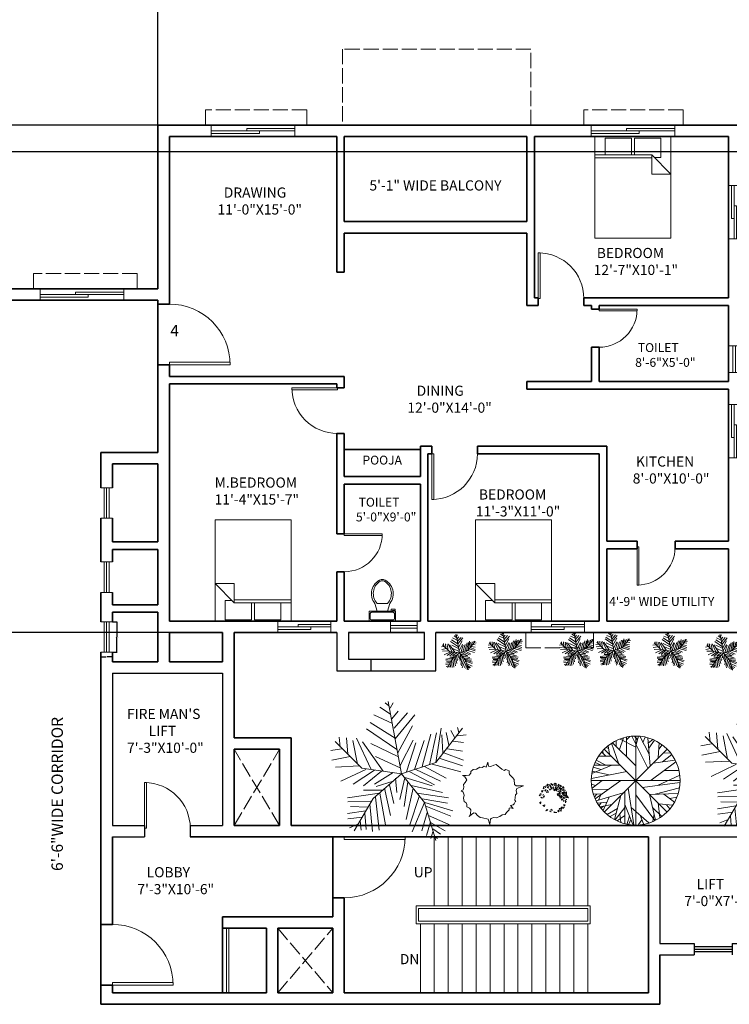
# Model space of a CAD drawing. Units: inches. Extents: x -69 to 2453, y 4803 to 7122.
# Tile 3 of 9: x 643 to 1203, y 5467 to 6243. Entities that reach past the tile are written whole.
import ezdxf

# ---------------------------------------------------------------- set-up
doc = ezdxf.new("R2010")
doc.units = ezdxf.units.IN
doc.linetypes.add('ACAD_ISO02W100', pattern=[15, 12, -3])
for name, color, linetype, lineweight in [('A-ANNO-DIMS', 2, 'Continuous', 18), ('A-ANNO-IDEN', 2, 'Continuous', 18), ('A-ANNO-TEXT', 7, 'Continuous', 18), ('A-AREA-IDEN', 7, 'Continuous', 18), ('A-DOOR', 3, 'Continuous', 18), ('A-FLOR-EVTR', 4, 'Continuous', 25), ('A-FLOR-FIXT', 9, 'Continuous', 18), ('A-FLOR-OPEN', 8, 'ACAD_ISO02W100', 13), ('A-FLOR-OVHD', 8, 'ACAD_ISO02W100', 13), ('A-FLOR-STRS', 4, 'Continuous', 18), ('A-FURN', 8, 'Continuous', 18), ('A-GLAZ', 244, 'Continuous', 18), ('A-WALL', 7, 'Continuous', 35), ('A-WALL-SRVC', 7, 'Continuous', 30), ('L-PLNT', 94, 'Continuous', 13)]:
    doc.layers.add(name, color=color, linetype=linetype, lineweight=lineweight)
doc.styles.get("Standard").update_dxf_attribs({"font": 'arial.ttf'})
doc.dimstyles.get("Standard").update_dxf_attribs({"dimtxt": 0.18, "dimasz": 0.18, "dimexe": 0.18, "dimexo": 0.0625, "dimgap": 0.09, "dimtad": 0, "dimtih": 1, "dimtoh": 1, "dimdec": 4, "dimzin": 0, "dimdsep": 46, "dimtxsty": 'Standard', "dimcen": 0.09, "dimadec": 0, "dimazin": 0, "dimtfac": 1, "dimtdec": 4, "dimtofl": 0, "dimtmove": 0, "dimatfit": 3, "dimfxl": 1, "dimtolj": 1, "dimtzin": 0, "dimarcsym": 0})

# ---------------------------------------------------------------- blocks, each defined once
blk = doc.blocks.new('*U7')
for p, q in [((0, 0), (0, -6)), ((-40, 0), (-40, -6))]:
    blk.add_line(p, q)
blk.add_lwpolyline([(0, 0), (0, 40), (-1.75, 40), (-1.75, 0)], close=True)
blk.add_arc((0, 0), 40, 90, 180)
blk = doc.blocks.new('*U5')
for p, q in [((0, 0), (0, -6)), ((40, 0), (40, -6))]:
    blk.add_line(p, q)
blk.add_lwpolyline([(0, 0), (0, 40), (1.75, 40), (1.75, 0)], close=True)
blk.add_arc((0, 0), 40, 0, 90)
blk = doc.blocks.new('*U4')
for p, q in [((0, 0), (0, -6)), ((-40, 0), (-40, -6))]:
    blk.add_line(p, q)
blk.add_lwpolyline([(0, 0), (0, 40), (-1.75, 40), (-1.75, 0)], close=True)
blk.add_arc((0, 0), 40, 90, 180)
blk = doc.blocks.new('*U3')
for p, q in [((0, 0), (0, 6)), ((40, 0), (40, 6))]:
    blk.add_line(p, q)
blk.add_lwpolyline([(0, 0), (0, -40), (1.75, -40), (1.75, 0)], close=True)
blk.add_arc((0, 0), 40, 270, 360)
blk = doc.blocks.new('*U8')
for p, q in [((0, 0), (0, 6)), ((40, 0), (40, 6))]:
    blk.add_line(p, q)
blk.add_lwpolyline([(0, 0), (0, -40), (1.75, -40), (1.75, 0)], close=True)
blk.add_arc((0, 0), 40, 270, 0)
blk = doc.blocks.new('*U21')
for p, q in [((-40, 0), (-40, -6)), ((0, 0), (0, -6))]:
    blk.add_line(p, q)
blk.add_lwpolyline([(0, 0), (0, 40), (-1.75, 40), (-1.75, 0)], close=True)
blk.add_arc((0, 0), 40, 90, 180)
blk = doc.blocks.new('*U23')
for p, q in [((0, 0), (0, -6)), ((40, 0), (40, -6))]:
    blk.add_line(p, q)
blk.add_lwpolyline([(0, 0), (0, 40), (1.75, 40), (1.75, 0)], close=True)
blk.add_arc((0, 0), 40, 0, 90)
blk = doc.blocks.new('*U27')
for points in [[(-5.78, 9.75), (-7.54, 9.23), (-8.01, 7.5), (-6.26, 8.45)], [(-4.43, 11.05), (-5.18, 10.36), (-3.96, 9.49), (-2.07, 10.36)], [(-4.84, 8.63), (-3.83, 7.85), (-4.03, 8.97)], [(-1.94, 9.49), (-2.48, 8.97), (-2.27, 8.54), (-1.8, 9.06)], [(-2, 11.66), (-1.6, 10.62), (-0.52, 10.1), (-0.18, 10.62), (-0.79, 10.96)], [(0.02, 9.06), (-1.33, 8.54), (-1.73, 7.16), (0.29, 7.76)], [(1.24, 12), (0.56, 11.31), (0.76, 10.01), (2.52, 11.05)], [(1.37, 8.54), (3.13, 8.8), (3.8, 7.85), (1.91, 7.76)], [(2.59, 9.93), (1.84, 9.75), (1.64, 9.23), (2.32, 9.41)], [(4.14, 11.14), (3.6, 10.01), (4, 9.23), (5.22, 8.71), (6.3, 9.41), (5.08, 10.19), (4.61, 10.01)], [(4.61, 8.28), (4.54, 7.76), (4.95, 7.59), (4.95, 8.28)], [(6.43, 7.94), (5.49, 7.68), (5.56, 6.21), (6.5, 6.64)], [(7.45, 9.32), (7.11, 7.94), (8.52, 7.94)], [(-11.32, 1.79), (-9.83, 2.31), (-9.63, 3.44), (-10.44, 3.52)], [(-8.21, 0.41), (-9.43, 0.32), (-9.83, 0.84)], [(-8.14, 6.03), (-9.36, 5.95), (-9.02, 4.73)], [(-8.21, 3.09), (-8.48, 2.31), (-7.87, 2.57)], [(-7, 1.79), (-7.94, 1.53), (-7.47, 0.49)], [(-5.78, 6.81), (-6.66, 6.21), (-6.52, 5.69)], [(-4.57, 6.38), (-5.45, 4.47), (-3.89, 4.82)], [(-2.88, 7.5), (-3.15, 6.64), (-2.27, 6.72)], [(0.76, 7.16), (0.09, 6.46), (1.1, 5.95)], [(1.71, 6.29), (1.71, 7.07), (2.65, 7.5), (2.11, 6.9)], [(2.52, 6.81), (2.52, 5.86), (4.41, 5.17), (4.61, 6.72)], [(3.53, 1.88), (2.86, 3.52), (3.8, 3.52)], [(4.41, 4.56), (4.27, 3.7), (5.49, 3.26)], [(4.27, 2.74), (5.29, 2.66), (4.41, 1.27)], [(5.83, 1.53), (5.02, 0.41), (5.49, -0.02), (6.5, 0.41)], [(5.49, 5.51), (5.42, 4.82), (6.16, 5.08)], [(7.51, 1.71), (6.91, 1.27), (6.23, 2.14)], [(8.12, 4.99), (7.11, 4.65), (6.5, 4.13), (7.38, 3.09), (8.12, 3.52), (7.65, 3.87)], [(7.85, 6.81), (7.18, 6.21), (9, 5.51), (9.33, 6.38)], [(8.12, 0.75), (7.51, 0.15), (8.93, -0.28), (9.13, 0.49)], [(8.19, 2.57), (7.92, 2.05), (8.66, 1.53)], [(8.73, 4.73), (8.19, 4.56), (8.39, 3.87), (8.59, 4.04)], [(10.28, 5.17), (9.2, 4.04), (9, 2.31), (10.48, 0.49), (11.76, 0.41), (10.35, 2.48), (9.33, 2.4), (10.28, 2.83)], [(-10.03, -2.71), (-10.64, -3.31), (-10.44, -4.44), (-9.9, -3.49)], [(-8.28, -5.73), (-6.79, -5.3), (-7, -6.51)], [(6.1, -8.94), (6.16, -7.21), (6.91, -6.69), (7.24, -7.38)], [(7.78, -0.8), (6.43, -1.5), (6.43, -0.72)], [(8.32, -1.75), (7.98, -2.53), (7.58, -2.1)], [(8.05, -8.07), (8.59, -7.12), (7.92, -7.55)], [(9.33, -5.13), (8.46, -6.25), (7.98, -5.22)], [(9.33, -1.75), (9.54, -3.74), (10.14, -2.53)], [(10.08, -0.63), (9.74, -1.32), (10.48, -0.89)], [(-4.84, -8.85), (-4.43, -9.45), (-5.99, -9.8)], [(-2.54, -10.06), (-3.02, -10.23), (-1.8, -10.67)], [(-2.34, -9.2), (-1.26, -8.5), (-0.99, -9.54)], [(0.22, -10.58), (0.83, -11.27), (2.59, -11.36)], [(4.07, -9.45), (3.53, -9.97), (4.07, -10.58), (4.61, -9.89)], [(5.29, -7.98), (4.61, -8.16), (5.02, -8.94)], [(6.03, -9.45), (5.42, -9.97), (6.16, -10.15)]]:
    blk.add_lwpolyline(points, close=True)
blk = doc.blocks.new('*U25')
for p, q in [((-10.186, 53.64), (-13.084, 55.962)), ((0, 0), (-10.5, 57)), ((-9.099, 51.782), (-6.563, 55.962)), ((-7.288, 39.707), (-21.778, 46.673)), ((-8.737, 47.138), (-17.069, 52.711)), ((-7.65, 43.423), (-2.578, 49.46)), ((-5.839, 35.992), (4.667, 48.067)), ((-5.114, 27.632), (10.463, 46.673)), ((-5.114, 28.097), (-24.676, 40.636)), ((-3.665, 19.273), (-27.574, 35.527)), ((-2.941, 16.486), (8.652, 37.85)), ((16.259, 5.805), (23.142, 31.348)), ((22.055, 7.198), (27.489, 32.277)), ((27, 9), (48, 36)), ((27.127, 9.056), (31.112, 35.992)), ((35.096, 32.741), (37.27, 22.524)), ((38.719, 34.134), (41.979, 28.561)), ((44.153, 36.456), (45.239, 32.741)), ((-31.5, 4.5), (-52.5, 25.5)), ((-48.585, 21.131), (-49.309, 29.026)), ((-43.513, 28.561), (-42.427, 15.558)), ((-38.442, 26.239), (-34.819, 7.663)), ((-35.544, 28.097), (-24.314, 3.947)), ((-14.533, 2.09), (-30.834, 25.31)), ((-24.314, 23.917), (-2.941, 13.7)), ((-1.129, 6.734), (9.014, 26.704)), ((3.942, 1.625), (11.187, 24.381)), ((10.101, 3.483), (17.708, 26.239)), ((31.836, 30.883), (32.561, 16.486)), ((40.53, 25.775), (48.862, 24.846)), ((43.791, 29.954), (51.036, 30.883)), ((-47.498, 19.737), (-55.83, 18.344)), ((33.285, 16.486), (48.862, 10.913)), ((36.183, 19.737), (48.137, 17.88)), ((-40.615, 13.7), (-55.105, 10.913)), ((-20.691, 13.7), (-1.129, 4.876)), ((0, 0), (27, 9)), ((29.662, 12.307), (48.137, 6.269)), ((-33.37, 6.269), (-52.207, 5.34)), ((-28.299, 3.483), (-47.86, -5.805)), ((-21.416, 3.018), (-38.079, -8.128)), ((0, 0), (-31.5, 4.5)), ((-15.982, 2.09), (-30.11, -9.521)), ((0, 0), (-22.5, -19.5)), ((-6.563, 1.161), (-21.416, -8.128)), ((0, 0), (18, -22.5)), ((6.478, 1.625), (26.04, -8.592)), ((11.187, 3.483), (30.749, -5.805)), ((18.07, 5.805), (35.096, -3.483)), ((24.229, 7.663), (46.688, 1.625)), ((-6.563, -5.805), (-19.967, -9.985)), ((-4.752, -3.483), (-3.665, -14.629)), ((2.493, -3.019), (-1.491, -20.202)), ((1.769, -2.555), (24.229, -9.521)), ((5.029, -6.27), (2.131, -25.775)), ((-17.431, -15.094), (-42.789, -18.809)), ((-15.257, -12.772), (-30.11, -12.772)), ((-17.069, -15.094), (-12.721, -40.172)), ((-13.446, -11.378), (-8.737, -32.741)), ((-9.461, -8.592), (-6.201, -23.453)), ((9.014, -11.378), (3.58, -35.992)), ((7.565, -9.056), (32.198, -14.629)), ((12.274, -15.094), (36.907, -18.809)), ((-24.314, -21.596), (-42.427, -22.06)), ((-22.5, -19.5), (-37.5, -45)), ((-20.691, -18.345), (-17.793, -44.352)), ((14.085, -16.951), (6.478, -40.172)), ((18.07, -22.524), (8.289, -45.745)), ((16.259, -19.738), (36.183, -22.989)), ((18, -22.5), (27, -52.5)), ((18.433, -22.524), (40.53, -29.026)), ((-28.299, -29.026), (-42.789, -31.348)), ((-26.849, -26.24), (-40.253, -25.775)), ((-29.023, -30.884), (-27.936, -43.887)), ((-25.038, -23.918), (-22.865, -45.281)), ((20.244, -30.419), (15.897, -44.816)), ((19.157, -25.311), (38.719, -33.206)), ((-30.834, -34.135), (-42.427, -35.528)), ((-32.646, -36.921), (-31.921, -44.352)), ((22.78, -37.85), (19.519, -48.532)), ((21.331, -32.741), (39.081, -40.636)), ((22.78, -38.314), (34.372, -44.816)), ((-34.457, -39.708), (-40.978, -42.494)), ((24.591, -45.745), (23.142, -50.854)), ((24.591, -43.423), (30.749, -47.603)), ((26.764, -49.925), (28.213, -50.854))]:
    blk.add_line(p, q)
blk = doc.blocks.new('*U28')
for p, q in [((-26.4472, 46.5894), (-26.2712, 53.8116)), ((-22.0458, 42.0753), (-16.5881, 57.6486)), ((-21.1656, 55.8436), (-0.0388, 45.0094)), ((-12.5388, 54.9406), (-7.9613, 59.4546)), ((-12.3627, 32.1443), (-12.5388, 58.7776)), ((-5.3205, 59.6806), (16.5105, 16.7963)), ((2.426, 54.9406), (-1.4472, 59.9056)), ((0, 59.9996), (0, -60)), ((0.4894, 48.6208), (3.6584, 59.6806)), ((18.2711, 35.5298), (5.419, 59.6806)), ((9.8203, 51.5549), (12.8133, 58.5516)), ((19.6795, 19.5047), (16.3344, 57.6486)), ((17.0387, 51.1035), (23.2006, 55.1666)), ((17.7429, 43.6552), (25.4894, 54.2636)), ((-43.8768, 36.4326), (-44.405, 40.2696)), ((42, 42), (-42, -42)), ((42, -42), (-42, 42)), ((-40.1797, 44.558), (-36.4825, 43.2038)), ((-37.0107, 47.0408), (-35.25, 35.5298)), ((-32.6092, 50.4264), (-23.2782, 23.5674)), ((-31.2008, 51.1035), (-0.2149, 20.1818)), ((31.6513, 50.8778), (30.2429, 30.5643)), ((31.1232, 42.5267), (35.8767, 48.1693)), ((-53.2078, 27.4044), (-40.1797, 20.859)), ((-49.8627, 32.8214), (-32.7853, 32.8214)), ((-45.8134, 38.2383), (-40.5318, 33.0471)), ((23.3767, 23.3417), (53.3063, 27.4044)), ((36.2288, 25.1474), (48.9049, 35.0784)), ((37.1091, 37.1098), (46.6161, 37.5612)), ((-32.2571, 20.6333), (-59.1937, 9.348)), ((-57.081, 17.9248), (-47.0458, 14.7649)), ((-56.0247, 20.859), (-20.8134, 20.859)), ((-54.7923, 24.4702), (-47.75, 21.0847)), ((54.3626, 25.3731), (20.9119, 0.3198)), ((38.5175, 13.4107), (58.2359, 13.6364)), ((-59.7219, 2.8025), (-12.0106, 12.0565)), ((-58.6656, 12.7336), (-35.9543, 7.5424)), ((-54.6162, -24.7335), (-20.2853, 0.0941)), ((29.3626, -6.6771), (59.4682, 7.091)), ((-60, 0), (60, 0)), ((-59.7219, -4.8714), (-54.2641, -6.6771)), ((-45.2853, -0.1316), (-59.0177, -10.0627)), ((-58.4895, -12.3197), (-36.4825, -11.6426)), ((-10.074, -10.0627), (-2.5036, -59.7178)), ((9.2922, -9.1598), (59.6443, -2.8401)), ((26.3697, -18.4138), (58.9401, -9.8369)), ((-57.081, -18.4138), (-45.2853, -17.9624)), ((-52.6797, -18.188), (-55.4966, -22.0251)), ((-53.2078, -27.442), (-16.7641, -16.6081)), ((-47.2219, -19.3166), (-50.2148, -26.3135)), ((-35.9543, -22.4765), (-44.0529, -40.5329)), ((-19.9331, -20.2194), (-28.5599, -52.721)), ((-14.8275, -15.0282), (-14.6515, -57.6865)), ((-0.0388, -19.0909), (25.8415, -53.8495)), ((18.6232, -18.6394), (26.7218, -53.3981)), ((18.7992, -18.6394), (57.3556, -17.2853)), ((38.1654, -18.188), (52.426, -29.0219)), ((45.9119, -24.0564), (55.595, -22.2508)), ((-38.9472, -29.0219), (-51.4472, -30.6018)), ((-46.5177, -30.1504), (-49.5106, -33.536)), ((-32.4331, -32.4075), (-48.1021, -35.5674)), ((-43.7008, -34.6645), (-46.6937, -37.373)), ((-24.6867, -37.8244), (-38.7712, -45.7241)), ((-14.6515, -36.2445), (-27.6797, -52.9467)), ((-14.6515, -32.1818), (-3.912, -59.4922)), ((-6.2008, -36.2445), (17.919, -57.0094)), ((22.8485, -36.4702), (35.3485, -48.4326)), ((30.419, -30.1504), (32.3556, -50.0125)), ((31.4753, -31.279), (49.6091, -33.3103)), ((41.5105, -32.6332), (46.088, -38.0501)), ((-26.2712, -43.9185), (-34.7219, -48.6583)), ((-14.6515, -47.3041), (-25.0388, -54.3009)), ((-21.5177, -45.4984), (-19.9331, -56.1065)), ((-8.4895, -47.5298), (-11.4825, -58.5893)), ((-6.3768, -52.721), (-9.3698, -58.815)), ((5.9471, -46.6269), (10.5246, -58.5893)), ((24.7852, -44.8213), (23.0246, -54.978)), ((8.4119, -53.1724), (3.8344, -59.4922))]:
    blk.add_line(p, q)
blk.add_circle((0, 0), 60)
blk = doc.blocks.new('*U29')
blk.add_lwpolyline([(-4.577, 66.508), (-7.629, 55.26), (-12.588, 57.705), (-17.165, 54.771), (-22.124, 55.26), (-29.372, 50.859), (-36.619, 50.37), (-41.578, 45.968), (-41.578, 42.056), (-45.393, 37.655), (-52.259, 36.677), (-60.651, 36.677), (-54.929, 33.743), (-51.115, 27.385), (-54.548, 21.028), (-58.362, 17.116), (-57.599, 11.248), (-58.744, 5.379), (-63.703, 2.445), (-59.125, 0), (-56.837, -6.846), (-58.362, -13.204), (-56.455, -20.539), (-52.259, -23.473), (-51.115, -27.386), (-51.115, -32.276), (-45.011, -35.21), (-41.96, -39.122), (-42.723, -47.925), (-45.393, -54.282), (-40.434, -49.392), (-35.475, -45.969), (-31.66, -46.947), (-27.083, -51.837), (-21.361, -56.238), (-16.021, -56.727), (-3.433, -60.151), (0, -71.887), (1.526, -60.151), (3.052, -58.194), (8.392, -56.238), (14.114, -56.727), (22.506, -54.282), (27.465, -50.37), (33.95, -49.392), (37.002, -44.991), (42.723, -39.611), (43.105, -35.699), (45.012, -34.721), (51.878, -36.188), (46.157, -29.342), (51.878, -28.364), (53.785, -25.919), (56.074, -21.517), (57.6, -20.539), (55.693, -18.094), (57.219, -5.868), (59.889, -2.934), (58.744, 3.423), (60.27, 7.824), (67.137, 11.248), (74.766, 14.182), (67.899, 13.693), (58.363, 13.693), (54.93, 16.627), (54.167, 27.874), (50.353, 32.276), (43.868, 39.122), (42.723, 42.545), (43.105, 47.436), (35.476, 49.881), (31.661, 47.925), (27.084, 50.859), (14.496, 61.128), (9.155, 59.661), (2.289, 56.727), (-3.051, 57.705)], close=True)
blk = doc.blocks.new('Bed - Queen')
for p, q in [((0, -80.00003), (0, 0)), ((0, 0), (59.99999, 0)), ((59.99999, 0), (59.99999, -80.00003)), ((7.99999, -1.2), (28.79998, -1.2)), ((7.99999, -14.4), (7.99999, -1.2)), ((28.79998, -1.2), (28.79998, -14.4)), ((31.19999, -1.2), (51.99999, -1.2)), ((31.19999, -14.4), (31.19999, -1.2)), ((51.99999, -1.2), (51.99999, -16.4)), ((0, -14.4), (44.8, -14.4)), ((59.99999, -29.6), (44.8, -14.4)), ((44.8, -14.4), (44.8, -29.6)), ((44.8, -16.8), (0, -16.8)), ((51.99999, -16.4), (46.79936, -16.4)), ((44.8, -29.6), (59.99999, -29.6)), ((59.99999, -80.00003), (0, -80.00003))]:
    blk.add_line(p, q)
blk = doc.blocks.new('*U33')
for p, q in [((9.5, -6), (9.5, -2)), ((-10, -8.5), (-8, -8.5)), ((-10, -9.5), (-10, -8.5)), ((-7, -9.5), (-10, -9.5)), ((-8, -8.5), (-8, -8)), ((-7, -8), (-7, -9.5)), ((-4, -8), (-6, -14)), ((4, -14), (-4, -14)), ((4, -8), (6, -14))]:
    blk.add_line(p, q)
blk.add_lwpolyline([(10.5, -8), (10.5, 0), (-10.5, 0), (-10.5, -8)], close=True)
for points in [[(-9.5, -2), (-9.5, -6)], [(8.5, -1), (-8.5, -1)], [(-8.5, -7), (8.5, -7)]]:
    blk.add_lwpolyline(points)
for centre, radius, start, end in [((-8.62, -1.88), 0.884, 81.8699, 188.1301), ((-8.62, -6.12), 0.884, 171.8699, 278.1301), ((8.62, -1.88), 0.884, 351.8699, 98.1301), ((8.62, -6.12), 0.884, 261.8699, 8.1301), ((3.52, -21.58), 12.17, 141.46911, 247.97143), ((4.2, -21.82), 11.33, 136.36773, 238.94682), ((-3.52, -21.58), 12.17, 292.02843, 38.53071), ((-4.2, -21.82), 11.33, 301.05301, 43.63209), ((0, -27.88), 4, 245.73182, 294.26817), ((0, -29), 4, 254.86053, 285.13947)]:
    blk.add_arc(centre, radius, start, end)
blk = doc.blocks.new('*U22')
for p, q in [((0, 0), (0, -6)), ((40, 0), (40, -6))]:
    blk.add_line(p, q)
blk.add_lwpolyline([(0, 0), (0, 40), (1.75, 40), (1.75, 0)], close=True)
blk.add_arc((0, 0), 40, 0, 90)
blk = doc.blocks.new('WINDOW-VENT-21IN')
for p, q in [((0, 5.5), (21, 5.5)), ((0, 3.5), (21, 3.5))]:
    blk.add_line(p, q)
blk.add_lwpolyline([(0, 9), (21, 9), (21, 0), (0, 0)], close=True)
blk = doc.blocks.new('WINDOW-SLIDING-42IN')
for p, q in [((2.5, 42), (2.5, 16)), ((4.5, 42), (4.5, 0)), ((4.5, 26), (6.5, 26)), ((6.5, 26), (6.5, 0)), ((4.5, 16), (2.5, 16))]:
    blk.add_line(p, q)
blk.add_lwpolyline([(0, 42), (9, 42), (9, 0), (0, 0)], close=True)
blk = doc.blocks.new('WINDOW-SLIDING-66IN')
for p, q in [((66, 4.5), (0, 4.5)), ((38, 2.5), (0, 2.5)), ((66, 6.5), (28, 6.5)), ((28, 4.5), (28, 6.5)), ((38, 4.5), (38, 2.5))]:
    blk.add_line(p, q)
blk.add_lwpolyline([(66, 9), (66, 0), (0, 0), (0, 9)], close=True)
blk = doc.blocks.new('LIFT-PASSENGER-84IN')
for p, q in [((0, 93), (84, 93)), ((0, 93), (0, 9)), ((84, 93), (84, 9)), ((0, 9), (27, 9)), ((27, 9), (27, 0)), ((57, 9), (57, 0)), ((57, 9), (84, 9)), ((27, 6.5), (57, 6.5)), ((27, 4.5), (57, 4.5)), ((27, 2.5), (57, 2.5))]:
    blk.add_line(p, q)
blk = doc.blocks.new('WINDOW-CORE-24IN')
for p, q in [((9, 24), (0, 24)), ((2.5, 24), (2.5, 0)), ((4.5, 24), (4.5, 0)), ((6.5, 24), (6.5, 0)), ((9, 0), (0, 0))]:
    blk.add_line(p, q)
blk = doc.blocks.new('*D73')
at = {"layer": 'A-ANNO-DIMS', "color": 0, "lineweight": -2, "transparency": 16777216}
for p, q in [((716.57, 5768.22), (720.29, 5768.22)), ((720.11, 5768.04), (720.11, 5756.4)), ((720.11, 5744.4), (720.11, 5756.03)), ((716.57, 5744.22), (720.29, 5744.22))]:
    blk.add_line(p, q, dxfattribs=at)
at = {"layer": 'A-ANNO-DIMS', "color": 0, "transparency": 16777216}
for points in [[(720.08, 5768.04), (720.14, 5768.04), (720.11, 5768.22)], [(720.08, 5744.4), (720.14, 5744.4), (720.11, 5744.22)]]:
    blk.add_solid(points, dxfattribs=at)
at = {"layer": 'Defpoints', "color": 0, "transparency": 16777216}
for p in [(716.51, 5768.22), (720.11, 5768.22), (716.51, 5744.22)]:
    blk.add_point(p, dxfattribs=at)
at = {"layer": 'A-ANNO-DIMS', "color": 0, "transparency": 16777216, "insert": (720.11, 5756.22), "char_height": 0.18, "attachment_point": 5}
blk.add_mtext('\\A1;CORE WINDOW 24 TYP.', dxfattribs=at)
blk = doc.blocks.new('*D74')
at = {"layer": 'A-ANNO-DIMS', "color": 0, "lineweight": -2, "transparency": 16777216}
for p, q in [((707.51, 5744.15), (707.51, 5740.44)), ((716.51, 5744.15), (716.51, 5740.44)), ((707.69, 5740.62), (711.55, 5740.62)), ((716.33, 5740.62), (712.47, 5740.62))]:
    blk.add_line(p, q, dxfattribs=at)
at = {"layer": 'A-ANNO-DIMS', "color": 0, "transparency": 16777216}
for points in [[(707.69, 5740.65), (707.69, 5740.59), (707.51, 5740.62)], [(716.33, 5740.65), (716.33, 5740.59), (716.51, 5740.62)]]:
    blk.add_solid(points, dxfattribs=at)
at = {"layer": 'Defpoints', "color": 0, "transparency": 16777216}
for p in [(707.51, 5744.22), (716.51, 5744.22), (716.51, 5740.62)]:
    blk.add_point(p, dxfattribs=at)
at = {"layer": 'A-ANNO-DIMS', "color": 0, "transparency": 16777216, "insert": (712.01, 5740.62), "char_height": 0.18, "attachment_point": 5}
blk.add_mtext('\\A1;9 TYP.', dxfattribs=at)
blk = doc.blocks.new('*D100')
at = {"layer": 'A-ANNO-DIMS', "color": 0, "lineweight": -2, "transparency": 16777216}
for p, q in [((752.51, 6159.78), (752.51, 7121.65)), ((752.69, 7121.47), (981.72, 7121.47)), ((1211.33, 7121.47), (982.3, 7121.47)), ((1211.51, 6159.78), (1211.51, 7121.65))]:
    blk.add_line(p, q, dxfattribs=at)
at = {"layer": 'A-ANNO-DIMS', "color": 0, "transparency": 16777216}
for points in [[(752.69, 7121.5), (752.69, 7121.44), (752.51, 7121.47)], [(1211.33, 7121.5), (1211.33, 7121.44), (1211.51, 7121.47)]]:
    blk.add_solid(points, dxfattribs=at)
at = {"layer": 'Defpoints', "color": 0, "transparency": 16777216}
for p in [(1211.51, 7121.47), (752.51, 6159.72), (1211.51, 6159.72)]:
    blk.add_point(p, dxfattribs=at)
at = {"layer": 'A-ANNO-DIMS', "color": 0, "transparency": 16777216, "insert": (982.01, 7121.47), "char_height": 0.18, "attachment_point": 5}
blk.add_mtext('\\A1;459', dxfattribs=at)
blk = doc.blocks.new('*D101')
at = {"layer": 'A-ANNO-DIMS', "color": 0, "lineweight": -2, "transparency": 16777216}
for p, q in [((752.45, 6159.72), (-69.42, 6159.72)), ((-69.24, 6159.54), (-69.24, 5959.9)), ((-69.24, 5759.9), (-69.24, 5959.53)), ((761.45, 5759.72), (-69.42, 5759.72))]:
    blk.add_line(p, q, dxfattribs=at)
at = {"layer": 'A-ANNO-DIMS', "color": 0, "transparency": 16777216}
for points in [[(-69.27, 6159.54), (-69.21, 6159.54), (-69.24, 6159.72)], [(-69.27, 5759.9), (-69.21, 5759.9), (-69.24, 5759.72)]]:
    blk.add_solid(points, dxfattribs=at)
at = {"layer": 'Defpoints', "color": 0, "transparency": 16777216}
for p in [(-69.24, 6159.72), (752.51, 6159.72), (761.51, 5759.72)]:
    blk.add_point(p, dxfattribs=at)
at = {"layer": 'A-ANNO-DIMS', "color": 0, "transparency": 16777216, "insert": (-69.24, 5959.72), "char_height": 0.18, "attachment_point": 5}
blk.add_mtext('\\A1;400', dxfattribs=at)
blk = doc.blocks.new('*D103')
at = {"layer": 'A-ANNO-DIMS', "color": 0, "lineweight": -2, "transparency": 16777216}
for p, q in [((1241.45, 6552.72), (-69.42, 6552.72)), ((-69.24, 6552.54), (-69.24, 6345.9)), ((-69.24, 6138.9), (-69.24, 6345.53)), ((1241.45, 6138.72), (-69.42, 6138.72))]:
    blk.add_line(p, q, dxfattribs=at)
at = {"layer": 'A-ANNO-DIMS', "color": 0, "transparency": 16777216}
for points in [[(-69.27, 6552.54), (-69.21, 6552.54), (-69.24, 6552.72)], [(-69.27, 6138.9), (-69.21, 6138.9), (-69.24, 6138.72)]]:
    blk.add_solid(points, dxfattribs=at)
at = {"layer": 'Defpoints', "color": 0, "transparency": 16777216}
for p in [(-69.24, 6552.72), (1241.51, 6552.72), (1241.51, 6138.72)]:
    blk.add_point(p, dxfattribs=at)
at = {"layer": 'A-ANNO-DIMS', "color": 0, "transparency": 16777216, "insert": (-69.24, 6345.72), "char_height": 0.18, "attachment_point": 5}
blk.add_mtext('\\A1;414', dxfattribs=at)

msp = doc.modelspace()

# ---------------------------------------------------------------- linework, layer by layer
at = {"layer": 'A-FLOR-EVTR'}
for p, q in [((716.51, 5727.72), (803.51, 5727.72)), ((716.51, 5727.72), (716.51, 5607.72)), ((803.51, 5727.72), (803.51, 5607.72)), ((716.51, 5607.72), (742.01, 5607.72)), ((742.01, 5607.72), (742.01, 5598.72)), ((778.01, 5607.72), (778.01, 5598.72)), ((778.01, 5607.72), (803.51, 5607.72)), ((716.51, 5598.72), (742.01, 5598.72)), ((1148.51, 5505.72), (1175.51, 5505.72))]:
    msp.add_line(p, q, dxfattribs=at)
at = {"layer": 'A-FLOR-OPEN'}
for p, q in [((812.51, 5607.72), (848.51, 5667.72)), ((848.51, 5607.72), (812.51, 5667.72)), ((847.01, 5526.72), (890.51, 5475.72)), ((847.01, 5475.72), (890.51, 5526.72))]:
    msp.add_line(p, q, dxfattribs=at)
at = {"layer": 'A-FLOR-OVHD'}
for p, q in [((1046.78, 6219.72), (897.98, 6219.72)), ((897.98, 6219.72), (897.98, 6159.72)), ((1046.78, 6159.72), (1046.78, 6219.72)), ((870.06, 6171.72), (790, 6171.72)), ((790, 6171.72), (790, 6159.72)), ((870.06, 6159.72), (870.06, 6171.72)), ((1166.93, 6171.72), (1088.39, 6171.72)), ((1088.39, 6171.72), (1088.39, 6159.72)), ((1166.93, 6159.72), (1166.93, 6171.72)), ((736.15, 6042.72), (654.3, 6042.72)), ((654.3, 6042.72), (654.3, 6030.72)), ((736.15, 6030.72), (736.15, 6042.72)), ((1042.65, 5759.72), (1042.65, 5747.72)), ((1096.06, 5747.72), (1096.06, 5759.72)), ((1042.65, 5747.72), (1096.06, 5747.72))]:
    msp.add_line(p, q, dxfattribs=at)
at = {"layer": 'A-FLOR-STRS'}
for p, q in [((970.51, 5598.72), (970.51, 5544.22)), ((981.51, 5598.72), (981.51, 5544.22)), ((992.51, 5598.72), (992.51, 5544.22)), ((1003.51, 5598.72), (1003.51, 5544.22)), ((1014.51, 5598.72), (1014.51, 5544.22)), ((1025.51, 5598.72), (1025.51, 5544.22)), ((1036.51, 5598.72), (1036.51, 5544.22)), ((1047.51, 5598.72), (1047.51, 5544.22)), ((1058.51, 5598.72), (1058.51, 5544.22)), ((1069.51, 5598.72), (1069.51, 5544.22)), ((1080.51, 5598.72), (1080.51, 5544.22)), ((1091.51, 5598.72), (1091.51, 5544.22)), ((1093.51, 5544.22), (956.13, 5544.22)), ((956.13, 5544.22), (956.13, 5530.22)), ((1091.51, 5542.22), (958.13, 5542.22)), ((958.13, 5542.22), (958.13, 5532.22)), ((1091.51, 5542.22), (1091.51, 5532.22)), ((1093.51, 5544.22), (1093.51, 5530.22)), ((1093.51, 5530.22), (956.13, 5530.22)), ((1091.51, 5532.22), (958.13, 5532.22)), ((959.51, 5530.22), (959.51, 5475.72)), ((970.51, 5530.22), (970.51, 5475.72)), ((981.51, 5530.22), (981.51, 5475.72)), ((992.51, 5530.22), (992.51, 5475.72)), ((1003.51, 5530.22), (1003.51, 5475.72)), ((1014.51, 5530.22), (1014.51, 5475.72)), ((1025.51, 5530.22), (1025.51, 5475.72)), ((1036.51, 5530.22), (1036.51, 5475.72)), ((1047.51, 5530.22), (1047.51, 5475.72)), ((1058.51, 5530.22), (1058.51, 5475.72)), ((1069.51, 5530.22), (1069.51, 5475.72)), ((1080.51, 5530.22), (1080.51, 5475.72)), ((1091.51, 5530.22), (1091.51, 5475.72))]:
    msp.add_line(p, q, dxfattribs=at)
at = {"layer": 'A-GLAZ'}
for p, q in [((806.51, 5526.72), (806.51, 5475.72)), ((808.51, 5526.72), (808.51, 5475.72))]:
    msp.add_line(p, q, dxfattribs=at)
at = {"layer": 'A-WALL'}
for p, q in [((752.51, 6159.72), (752.51, 6030.72)), ((752.51, 6159.72), (1241.51, 6159.72)), ((761.51, 6150.72), (761.51, 6018.72)), ((761.51, 6150.72), (893.51, 6150.72)), ((893.51, 6150.72), (893.51, 6043.8)), ((899.51, 6150.72), (899.51, 6083.72)), ((899.51, 6150.72), (1043.51, 6150.72)), ((1043.51, 6150.72), (1043.51, 6083.72)), ((1049.51, 6150.72), (1049.51, 6023.72)), ((1049.51, 6150.72), (1202.51, 6150.72)), ((1202.51, 6150.72), (1202.51, 6023.72)), ((899.51, 6083.72), (1043.51, 6083.72)), ((899.51, 6074.72), (1043.51, 6074.72)), ((899.51, 6074.72), (899.51, 6043.8)), ((1043.51, 6074.72), (1043.51, 6017.72)), ((899.51, 6043.8), (893.51, 6043.8)), ((623.51, 6030.72), (752.51, 6030.72)), ((1049.51, 6023.72), (1052.51, 6023.72)), ((1052.51, 6023.72), (1052.51, 6017.72)), ((1088.51, 6023.72), (1088.51, 6017.72)), ((1088.51, 6023.72), (1202.51, 6023.72)), ((632.51, 6021.72), (752.51, 6021.72)), ((752.51, 6021.72), (752.51, 5901.72)), ((752.51, 6018.72), (761.51, 6018.72)), ((1043.51, 6017.72), (1052.51, 6017.72)), ((1088.51, 6017.72), (1094.51, 6017.72)), ((1094.51, 6017.72), (1094.51, 6014.72)), ((1100.51, 6017.72), (1100.51, 6014.72)), ((1100.51, 6017.72), (1202.51, 6017.72)), ((1202.51, 6017.72), (1202.51, 5957.72)), ((1094.51, 6014.72), (1100.51, 6014.72)), ((1094.51, 5984.72), (1100.51, 5984.72)), ((1094.51, 5984.72), (1094.51, 5957.72)), ((1100.51, 5984.72), (1100.51, 5957.72)), ((752.51, 5970.72), (761.51, 5970.72)), ((761.51, 5970.72), (761.51, 5961.72)), ((761.51, 5961.72), (899.51, 5961.72)), ((899.51, 5961.72), (899.51, 5952.72)), ((761.51, 5955.72), (893.51, 5955.72)), ((761.51, 5955.72), (761.51, 5768.72)), ((893.51, 5955.72), (893.51, 5952.72)), ((1043.51, 5957.72), (1094.51, 5957.72)), ((1043.51, 5957.72), (1043.51, 5951.72)), ((1100.51, 5957.72), (1202.51, 5957.72)), ((893.51, 5952.72), (899.51, 5952.72)), ((1043.51, 5951.72), (1202.51, 5951.72)), ((1202.51, 5951.72), (1202.51, 5831.72)), ((893.51, 5916.72), (899.51, 5916.72)), ((893.51, 5916.72), (893.51, 5837.72)), ((899.51, 5916.72), (899.51, 5882.72)), ((707.51, 5901.72), (752.51, 5901.72)), ((707.51, 5901.72), (707.51, 5873.96)), ((959.51, 5904.12), (899.51, 5904.12)), ((959.51, 5906.72), (959.51, 5882.72)), ((959.51, 5906.72), (968.51, 5906.72)), ((965.51, 5900.72), (965.51, 5768.72)), ((965.51, 5900.72), (968.51, 5900.72)), ((968.51, 5900.72), (968.51, 5906.72)), ((1004.51, 5900.72), (1004.51, 5906.72)), ((1004.51, 5906.72), (1106.51, 5906.72)), ((1004.51, 5900.72), (1100.51, 5900.72)), ((1100.51, 5900.72), (1100.51, 5768.72)), ((1106.51, 5906.72), (1106.51, 5831.72)), ((716.51, 5892.72), (752.51, 5892.72)), ((716.51, 5892.72), (716.51, 5873.96)), ((752.51, 5892.72), (752.51, 5831.21)), ((899.51, 5882.72), (959.51, 5882.72)), ((899.51, 5876.72), (959.51, 5876.72)), ((899.51, 5876.72), (899.51, 5837.72)), ((959.51, 5876.72), (959.51, 5768.72)), ((707.51, 5849.96), (707.51, 5815.46)), ((716.51, 5849.96), (716.51, 5831.21)), ((899.51, 5837.72), (893.51, 5837.72)), ((716.51, 5831.21), (752.51, 5831.21)), ((1106.51, 5831.72), (1130.51, 5831.72)), ((1130.51, 5825.72), (1130.51, 5831.72)), ((1160.51, 5825.72), (1160.51, 5831.72)), ((1160.51, 5831.72), (1202.51, 5831.72)), ((716.51, 5825.21), (752.51, 5825.21)), ((716.51, 5825.21), (716.51, 5815.46)), ((752.51, 5825.21), (752.51, 5781.72)), ((1106.51, 5825.72), (1130.51, 5825.72)), ((1106.51, 5825.72), (1106.51, 5768.72)), ((1160.51, 5825.72), (1202.51, 5825.72)), ((1202.51, 5825.72), (1202.51, 5768.72)), ((899.51, 5807.72), (893.51, 5807.72)), ((893.51, 5807.72), (893.51, 5768.72)), ((899.51, 5807.72), (899.51, 5768.72)), ((707.51, 5791.46), (707.51, 5768.22)), ((716.51, 5791.46), (716.51, 5781.72)), ((716.51, 5781.72), (752.51, 5781.72)), ((716.51, 5775.72), (752.51, 5775.72)), ((716.51, 5775.72), (716.51, 5768.22)), ((752.51, 5775.72), (752.51, 5736.72)), ((761.51, 5768.72), (893.51, 5768.72)), ((899.51, 5768.72), (959.51, 5768.72)), ((965.51, 5768.72), (1100.51, 5768.72)), ((1106.51, 5768.72), (1202.51, 5768.72)), ((761.51, 5759.72), (803.51, 5759.72)), ((761.51, 5759.72), (761.51, 5736.72)), ((803.51, 5759.72), (803.51, 5736.72)), ((812.51, 5759.72), (812.51, 5676.72)), ((812.51, 5759.72), (893.74, 5759.72)), ((902.74, 5759.72), (962.78, 5759.72)), ((971.78, 5759.72), (1211.51, 5759.72)), ((707.51, 5744.22), (707.51, 5466.72)), ((716.51, 5744.22), (716.51, 5736.72)), ((716.51, 5736.72), (752.51, 5736.72)), ((761.51, 5736.72), (803.51, 5736.72)), ((812.51, 5676.72), (857.51, 5676.72)), ((857.51, 5676.72), (857.51, 5607.72)), ((812.51, 5667.72), (848.51, 5667.72)), ((812.51, 5667.72), (812.51, 5607.72)), ((848.51, 5667.72), (848.51, 5607.72)), ((812.51, 5607.72), (848.51, 5607.72)), ((857.51, 5607.72), (1427.51, 5607.72)), ((716.51, 5598.72), (716.51, 5529.72)), ((778.01, 5598.72), (1139.51, 5598.72)), ((890.51, 5598.72), (890.51, 5535.72)), ((1139.51, 5598.72), (1139.51, 5475.72)), ((890.51, 5550.72), (899.51, 5550.72)), ((899.51, 5550.72), (899.51, 5475.72)), ((803.51, 5535.72), (803.51, 5475.72)), ((803.51, 5535.72), (890.51, 5535.72)), ((716.51, 5529.72), (707.51, 5529.72)), ((803.51, 5526.72), (838.01, 5526.72)), ((838.01, 5526.72), (838.01, 5475.72)), ((847.01, 5526.72), (847.01, 5475.72)), ((847.01, 5526.72), (890.51, 5526.72)), ((890.51, 5526.72), (890.51, 5475.72)), ((1148.51, 5505.72), (1148.51, 5466.72)), ((716.51, 5481.72), (707.51, 5481.72)), ((716.51, 5481.72), (716.51, 5475.72)), ((716.51, 5475.72), (838.01, 5475.72)), ((847.01, 5475.72), (890.51, 5475.72)), ((899.51, 5475.72), (1139.51, 5475.72)), ((707.51, 5466.72), (1148.51, 5466.72))]:
    msp.add_line(p, q, dxfattribs=at)
at = {"layer": 'A-WALL-SRVC'}
for p, q in [((893.74, 5759.72), (893.74, 5729.72)), ((902.74, 5759.72), (902.74, 5738.72)), ((962.78, 5738.72), (962.78, 5759.72)), ((971.78, 5729.72), (971.78, 5759.72)), ((902.74, 5738.72), (962.78, 5738.72)), ((920.42, 5738.72), (920.42, 5729.72)), ((893.74, 5729.72), (971.78, 5729.72))]:
    msp.add_line(p, q, dxfattribs=at)

# ---------------------------------------------------------------- block references
at = {"layer": 'A-DOOR'}
for name, p, xscale, yscale, zscale in [('*U5', (1052.51, 6023.12), 0.9, 0.9, 0.9), ('*U3', (968.51, 5900.72), 0.9, 0.9, 0.9), ('*U22', (742.01, 5605.47), 0.8992305598406893, 0.8992305598406893, 0.8992305598406893)]:
    msp.add_blockref(name, p, dxfattribs=dict(at, xscale=xscale, yscale=yscale, zscale=zscale))
for name, p, xscale, yscale, zscale, rotation in [('*U7', (761.51, 5970.72), 1.199999999999977, 1.199999999999977, 1.199999999999977, 270.0000000000001), ('*U5', (1100.51, 6014.72), 0.75, 0.75, 0.75, 270.0000000000001), ('*U8', (894.11, 5952.72), 0.9, 0.9, 0.9, 270), ('*U5', (899.51, 5837.72), 0.75, 0.75, 0.75, 270.0000000000001), ('*U4', (1130.51, 5827.22), 0.75, 0.75, 0.75, 180), ('*U23', (899.51, 5598.72), 1.199999999999977, 1.199999999999977, 1.199999999999977, 270.0000000000001), ('*U21', (716.51, 5481.72), 1.199999999999977, 1.199999999999977, 1.199999999999977, 270.0000000000001)]:
    msp.add_blockref(name, p, dxfattribs=dict(at, xscale=xscale, yscale=yscale, zscale=zscale, rotation=rotation))
at = {"layer": 'A-FLOR-EVTR'}
msp.add_blockref('LIFT-PASSENGER-84IN', (1148.51, 5505.72), dxfattribs=at)
at = {"layer": 'A-FLOR-FIXT', "rotation": 180}
msp.add_blockref('*U33', (929.51, 5768.72), dxfattribs=at)
at = {"layer": 'A-FURN'}
msp.add_blockref('Bed - Queen', (1097.21, 6150.72), dxfattribs=at)
at = {"layer": 'A-FURN', "rotation": 180}
for p in [(857.51, 5768.72), (1063.01, 5768.72)]:
    msp.add_blockref('Bed - Queen', p, dxfattribs=at)
at = {"layer": 'A-GLAZ'}
for name, p in [('WINDOW-SLIDING-66IN', (794.51, 6150.72)), ('WINDOW-SLIDING-66IN', (1094.21, 6150.72)), ('WINDOW-SLIDING-42IN', (1202.51, 6070.25)), ('WINDOW-SLIDING-66IN', (659.51, 6021.72)), ('WINDOW-SLIDING-42IN', (1202.51, 5897.44)), ('WINDOW-CORE-24IN', (707.51, 5849.96)), ('WINDOW-CORE-24IN', (707.51, 5791.46)), ('WINDOW-CORE-24IN', (707.51, 5744.22)), ('WINDOW-VENT-21IN', (936.02, 5759.72))]:
    msp.add_blockref(name, p, dxfattribs=at)
for name, p, rotation in [('WINDOW-VENT-21IN', (1202.51, 5985.87), 269.999999999998), ('WINDOW-SLIDING-42IN', (847, 5768.72), 269.9999999999962), ('WINDOW-SLIDING-42IN', (1046.93, 5768.72), 269.9999999999984)]:
    msp.add_blockref(name, p, dxfattribs=dict(at, rotation=rotation))
at = {"layer": 'L-PLNT'}
for name, p, xscale, yscale, zscale in [('*U25', (1027.14, 5745.14), 0.2549892445070385, 0.2549892445070385, 0.2549892445070385), ('*U25', (1083.47, 5745.14), 0.2549892445070385, 0.2549892445070385, 0.2549892445070385), ('*U25', (1112.21, 5745.65), 0.2549892445070385, 0.2549892445070385, 0.2549892445070385), ('*U25', (1157.27, 5745.14), 0.2549892445070385, 0.2549892445070385, 0.2549892445070385), ('*U25', (990.41, 5743.72), 0.2549892445070385, 0.2549892445070385, 0.2549892445070385), ('*U25', (1198.79, 5743.62), 0.2549892445070385, 0.2549892445070385, 0.2549892445070385), ('*U28', (1129.41, 5643.11), 0.5842112454010082, 0.5842112454010082, 0.5842112454010082), ('*U29', (1014.26, 5634), 0.356051830328967, 0.356051830328967, 0.356051830328967)]:
    msp.add_blockref(name, p, dxfattribs=dict(at, xscale=xscale, yscale=yscale, zscale=zscale))
for name, p in [('*U25', (944.71, 5648.35)), ('*U25', (1236.73, 5652.21)), ('*U27', (1064.49, 5629.15))]:
    msp.add_blockref(name, p, dxfattribs=at)

# ---------------------------------------------------------------- texts
at = {"layer": 'A-ANNO-IDEN', "insert": (762.21, 6002.27), "char_height": 8, "attachment_point": 1}
msp.add_mtext_dynamic_manual_height_columns('{\\H1.125x;4} ', width=10.4994, gutter_width=12.5, heights=[0], dxfattribs=at)
at = {"layer": 'A-ANNO-TEXT', "char_height": 8, "attachment_point": 1}
for s, insert in [('UP', (954.33, 5574.84)), ('DN ', (943.33, 5506.34))]:
    msp.add_mtext_dynamic_manual_height_columns(s, width=16.1756, gutter_width=12.5, heights=[0], dxfattribs=dict(at, insert=insert))
at = {"layer": 'A-AREA-IDEN', "attachment_point": 1}
for s, width, insert, char_height in [('5\'-1" WIDE BALCONY', 114.3745, (919.32, 6116.25), 8), ('  DRAWING\\P11\'-0"X15\'-0"', 66.0939, (799.55, 6110.63), 8), (' BEDROOM\\P12\'-7"X10\'-1"', 64.9911, (1096.24, 6062.99), 8), (' TOILET\\P8\'-6"X5\'-0"', 45.2514, (1128.97, 5987.92), 7), ('   DINING\\P12\'-0"X14\'-0"', 63.2359, (949.27, 5954.4), 8), ('POOJA', 33.9191, (913.86, 5899.2), 7), (' KITCHEN\\P8\'-0"X10\'-0"', 58.1282, (1127.07, 5898.59), 8), ('M.BEDROOM\\P11\'-4"X15\'-7"', 69.6032, (797.22, 5882.02), 8), (' BEDROOM\\P11\'-3"X11\'-0"', 64.9911, (1003.28, 5872.61), 8), (' TOILET\\P5\'-0"X9\'-0"', 45.2002, (908.7, 5866.06), 7), ('4\'-9" WIDE UTILITY', 87.9123, (1108.46, 5787.78), 7), ('FIRE MAN\'S         LIFT 7\'-3"X10\'-0"', 62.3788, (728.07, 5699.62), 8), ('   LOBBY\\P7\'-3"X10\'-6"', 57.1555, (736.27, 5574.84), 8), ('    LIFT\\P7\'-0"X7\'-0"', 51.7015, (1167.69, 5565.47), 8)]:
    msp.add_mtext_dynamic_manual_height_columns(s, width=width, gutter_width=12.5, heights=[0], dxfattribs=dict(at, insert=insert, char_height=char_height))
at = {"layer": 'A-AREA-IDEN', "insert": (668.51, 5571.82), "char_height": 9, "attachment_point": 1, "rotation": 90}
msp.add_mtext_dynamic_manual_height_columns('6\'-6"WIDE CORRIDOR', width=131.0566, gutter_width=12.5, heights=[0], dxfattribs=at)

# ---------------------------------------------------------------- dimensions: what is measured, and where the dimension line sits
at = {"layer": 'A-ANNO-DIMS'}
dim = msp.add_linear_dim(base=(1211.51, 7121.47), p1=(752.51, 6159.72), p2=(1211.51, 6159.72), dimstyle='Standard', override={"dimdec": 0, "dimlfac": 1, "dimrnd": 0, "dimzin": 0, "dimdsep": 46, "dimlunit": 2}, dxfattribs=at)
dim.commit()
dim.dimension.update_dxf_attribs({"geometry": '*D100', "text_midpoint": (982.01, 7121.47)})
for base, p1, p2, picture, middle in [((-69.24, 6552.72), (1241.51, 6138.72), (1241.51, 6552.72), '*D103', (-69.24, 6345.72)), ((-69.24, 6159.72), (761.51, 5759.72), (752.51, 6159.72), '*D101', (-69.24, 5959.72))]:
    dim = msp.add_linear_dim(base=base, p1=p1, p2=p2, angle=90, dimstyle='Standard', override={"dimdec": 0, "dimlfac": 1, "dimrnd": 0, "dimzin": 0, "dimdsep": 46, "dimlunit": 2}, dxfattribs=at)
    dim.commit()
    dim.dimension.update_dxf_attribs({"geometry": picture, "text_midpoint": middle})
dim = msp.add_linear_dim(base=(720.11, 5768.22), p1=(716.51, 5744.22), p2=(716.51, 5768.22), angle=90, text='CORE WINDOW <> TYP.', dimstyle='Standard', override={"dimdec": 0, "dimlfac": 1, "dimrnd": 0, "dimzin": 0, "dimdsep": 46, "dimlunit": 2}, dxfattribs=at)
dim.commit()
dim.dimension.update_dxf_attribs({"geometry": '*D73', "text_midpoint": (720.11, 5756.22)})
dim = msp.add_linear_dim(base=(716.51, 5740.62), p1=(707.51, 5744.22), p2=(716.51, 5744.22), text='<> TYP.', dimstyle='Standard', override={"dimdec": 0, "dimlfac": 1, "dimrnd": 0, "dimzin": 0, "dimdsep": 46, "dimlunit": 2}, dxfattribs=at)
dim.commit()
dim.dimension.update_dxf_attribs({"geometry": '*D74', "text_midpoint": (712.01, 5740.62)})

doc.saveas('drawing.dxf')
